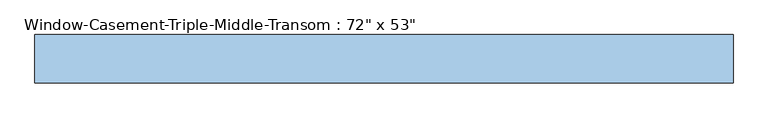
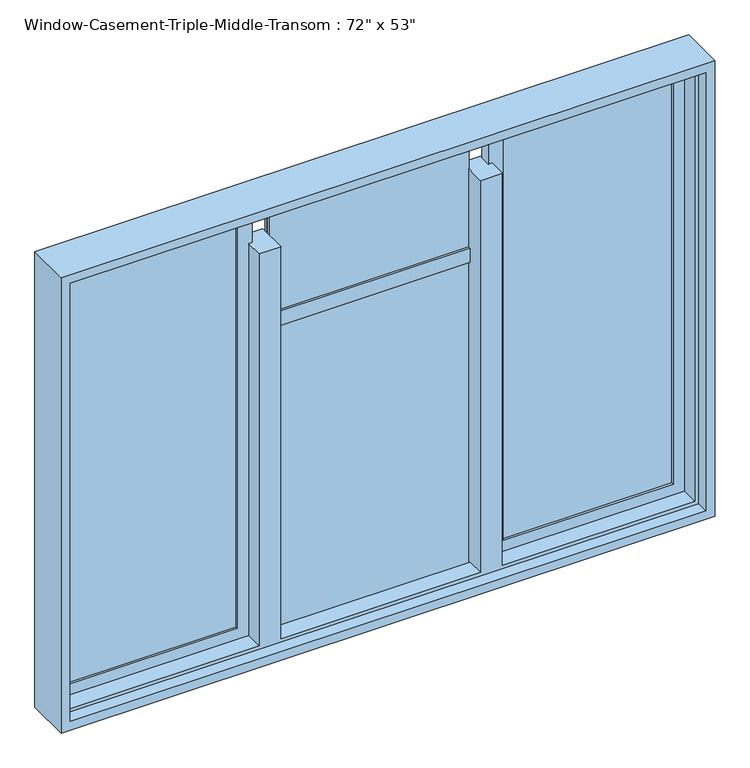
"""IFC4 building model written with IfcOpenShell, lengths in millimetres: window geometry."""

from ifc_helpers import new_model, si_unit, frame, origin, place, context, project, spatial, polyline, outline, extrude, faceted_brep, source, transform, mapped, element, save


def window_d2cb8397(model_context):
    return source(origin(), model_context, "Body", "SolidModel", [
        extrude(outline(polyline([(2235.2, 330.2), (939.8, 330.2), (939.8, 889.0), (2235.2, 889.0), (2235.2, 330.2)]), holes=[polyline([(2193.3296875, 847.1296875), (981.6703125, 847.1296875), (981.6703125, 372.0703125), (2193.3296875, 372.0703125), (2193.3296875, 847.1296875)])]), frame((0.0, 22.225, 0.0), z_axis=(0.0, 1.0, 0.0), x_axis=(0.0, 0.0, 1.0)), (0.0, 0.0, 1.0), 31.75),
        extrude(outline(polyline([(2235.2, -889.0), (939.8, -889.0), (939.8, -330.2), (2235.2, -330.2), (2235.2, -889.0)]), holes=[polyline([(2193.3296875, -372.0703125), (981.6703125, -372.0703125), (981.6703125, -847.1296875), (2193.3296875, -847.1296875), (2193.3296875, -372.0703125)])]), frame((0.0, 22.225, 0.0), z_axis=(0.0, 1.0, 0.0), x_axis=(0.0, 0.0, 1.0)), (0.0, 0.0, 1.0), 31.75),
        extrude(outline(polyline([(-372.0703125, 47.625), (-372.0703125, 41.275), (-847.1296875, 41.275), (-847.1296875, 47.625), (-372.0703125, 47.625)])), frame((0.0, 0.0, 949.9203125), z_axis=(0.0, 0.0, 1.0), x_axis=(1.0, 0.0, 0.0)), (0.0, 0.0, 1.0), 1275.159375),
        extrude(outline(polyline([(-372.0703125, 34.925), (-372.0703125, 28.575), (-847.1296875, 28.575), (-847.1296875, 34.925), (-372.0703125, 34.925)])), frame((0.0, 0.0, 949.9203125), z_axis=(0.0, 0.0, 1.0), x_axis=(1.0, 0.0, 0.0)), (0.0, 0.0, 1.0), 1275.159375),
        extrude(outline(polyline([(847.1296875, 47.625), (847.1296875, 41.275), (372.0703125, 41.275), (372.0703125, 47.625), (847.1296875, 47.625)])), frame((0.0, 0.0, 949.9203125), z_axis=(0.0, 0.0, 1.0), x_axis=(1.0, 0.0, 0.0)), (0.0, 0.0, 1.0), 1275.159375),
        extrude(outline(polyline([(847.1296875, 34.925), (847.1296875, 28.575), (372.0703125, 28.575), (372.0703125, 34.925), (847.1296875, 34.925)])), frame((0.0, 0.0, 949.9203125), z_axis=(0.0, 0.0, 1.0), x_axis=(1.0, 0.0, 0.0)), (0.0, 0.0, 1.0), 1275.159375),
        extrude(outline(polyline([(279.4, 53.975), (279.4, 22.225), (-279.4, 22.225), (-279.4, 53.975), (279.4, 53.975)])), frame((0.0, 0.0, 1835.8048438), z_axis=(0.0, 0.0, 1.0), x_axis=(1.0, 0.0, 0.0)), (0.0, 0.0, 1.0), 41.8703125),
        extrude(outline(polyline([(279.4, 47.625), (279.4, 41.275), (-279.4, 41.275), (-279.4, 47.625), (279.4, 47.625)])), frame((0.0, 0.0, 939.8), z_axis=(0.0, 0.0, 1.0), x_axis=(1.0, 0.0, 0.0)), (0.0, 0.0, 1.0), 896.0048437),
        extrude(outline(polyline([(279.4, 34.925), (279.4, 28.575), (-279.4, 28.575), (-279.4, 34.925), (279.4, 34.925)])), frame((0.0, 0.0, 939.8), z_axis=(0.0, 0.0, 1.0), x_axis=(1.0, 0.0, 0.0)), (0.0, 0.0, 1.0), 896.0048437),
        extrude(outline(polyline([(279.4, 47.625), (279.4, 41.275), (-279.4, 41.275), (-279.4, 47.625), (279.4, 47.625)])), frame((0.0, 0.0, 1877.6751563), z_axis=(0.0, 0.0, 1.0), x_axis=(1.0, 0.0, 0.0)), (0.0, 0.0, 1.0), 357.5248438),
        extrude(outline(polyline([(279.4, 34.925), (279.4, 28.575), (-279.4, 28.575), (-279.4, 34.925), (279.4, 34.925)])), frame((0.0, 0.0, 1877.6751563), z_axis=(0.0, 0.0, 1.0), x_axis=(1.0, 0.0, 0.0)), (0.0, 0.0, 1.0), 357.5248438),
        faceted_brep([(-889.0, 22.225, 2235.2), (-889.0, 63.5, 2235.2), (889.0, 63.5, 2235.2), (889.0, 22.225, 2235.2), (-878.8796875, -28.575, 2225.0796875), (-878.8796875, 22.225, 2225.0796875), (878.8796875, 22.225, 2225.0796875), (878.8796875, -28.575, 2225.0796875), (-889.0, -63.5, 2235.2), (-889.0, -28.575, 2235.2), (889.0, -28.575, 2235.2), (889.0, -63.5, 2235.2), (-914.4, 63.5, 2260.6), (-914.4, -63.5, 2260.6), (914.4, -63.5, 2260.6), (914.4, 63.5, 2260.6), (889.0, 63.5, 939.8), (889.0, 22.225, 939.8), (878.8796875, 22.225, 949.9203125), (878.8796875, -28.575, 949.9203125), (889.0, -28.575, 939.8), (889.0, -63.5, 939.8), (914.4, -63.5, 914.4), (914.4, 63.5, 914.4), (330.2, 22.225, 939.8), (-889.0, 63.5, 939.8), (-889.0, 22.225, 939.8), (-330.2, 22.225, 939.8), (-330.2, 60.325, 939.8), (-279.4, 60.325, 939.8), (-279.4, 22.225, 939.8), (279.4, 22.225, 939.8), (279.4, 60.325, 939.8), (330.2, 60.325, 939.8), (340.3203125, 22.225, 949.9203125), (340.3203125, -28.575, 949.9203125), (-878.8796875, 22.225, 949.9203125), (-878.8796875, -28.575, 949.9203125), (-340.3203125, -28.575, 949.9203125), (-340.3203125, 22.225, 949.9203125), (279.4, 22.225, 949.9203125), (-279.4, 22.225, 949.9203125), (-279.4, -28.575, 949.9203125), (279.4, -28.575, 949.9203125), (-889.0, -28.575, 939.8), (-889.0, -63.5, 939.8), (-914.4, -63.5, 914.4), (-914.4, 63.5, 914.4), (330.2, 22.225, 2108.2), (340.3203125, 22.225, 2108.2), (-340.3203125, 22.225, 2108.2), (-330.2, 22.225, 2108.2), (-279.4, 60.325, 2108.2), (-330.2, 60.325, 2108.2), (-340.3203125, -28.575, 2108.2), (-279.4, -28.575, 2108.2), (330.2, 60.325, 2108.2), (279.4, 60.325, 2108.2), (279.4, -28.575, 2108.2), (340.3203125, -28.575, 2108.2)], [[[0, 1, 2, 3]], [[4, 5, 6, 7]], [[8, 9, 10, 11]], [[12, 13, 14, 15]], [[3, 2, 16, 17]], [[7, 6, 18, 19]], [[11, 10, 20, 21]], [[15, 14, 22, 23]], [[24, 17, 16, 25, 26, 27, 28, 29, 30, 31, 32, 33]], [[19, 18, 34, 35]], [[36, 37, 38, 39]], [[40, 41, 42, 43]], [[21, 20, 44, 45]], [[23, 22, 46, 47]], [[1, 0, 26, 25]], [[0, 3, 17, 24, 48, 49, 34, 18, 6, 5, 36, 39, 50, 51, 27, 26]], [[41, 40, 31, 30]], [[5, 4, 37, 36]], [[9, 8, 45, 44]], [[14, 13, 46, 22], [8, 11, 21, 45]], [[13, 12, 47, 46]], [[12, 15, 23, 47], [2, 1, 25, 16]], [[52, 53, 51, 50, 54, 55]], [[56, 57, 58, 59, 49, 48]], [[53, 52, 29, 28]], [[27, 51, 53, 28]], [[52, 55, 42, 41, 30, 29]], [[57, 56, 33, 32]], [[58, 57, 32, 31, 40, 43]], [[56, 48, 24, 33]], [[54, 50, 39, 38]], [[49, 59, 35, 34]], [[10, 9, 44, 20], [4, 7, 19, 35, 59, 58, 43, 42, 55, 54, 38, 37]]]),
    ])


if __name__ == "__main__":
    model = new_model("IFC4")
    model_context = context("Model", 3, world=origin())
    ifc_project = project(units=[si_unit("LENGTHUNIT", "METRE", prefix="MILLI")], contexts=[model_context])
    site = spatial("IfcSite", under=ifc_project)
    building = spatial("IfcBuilding", under=site)
    placement = place(None, origin())
    window_shape = window_d2cb8397(model_context)
    element("IfcWindow", 1, ObjectType="Window-Casement-Triple-Middle-Transom : 72\" x 53\"", at=placement, inside=building, context=model_context, shape_type="MappedRepresentation", body=[
        mapped(window_shape, transform((0.0, 0.0, 0.0), x_axis=(1.0, 0.0, 0.0), y_axis=(0.0, 1.0, 0.0), z_axis=(0.0, 0.0, 1.0))),
    ])
    save(model, "model.ifc")

# Revit data of these elements
# Type "Window-Casement-Triple-Middle-Transom : 72\" x 53\""
#   Type Mark = "52"
#   Fire Rating = "0.5h"
#   Assembly Code = "B2020100"
#   Analytic Construction = "Double glazing - domestic"
#   Window Width = 2' - 0"
#   Window Inset [instance default] = 0' - 0 5/8"
#   Wall Thickness [instance default] = 0' - 6"
#   Visual Light Transmittance = 0.81
#   Transom Height Ratio = 0.3
#   Thermal Resistance (R) = 0.319569 (m²·K)/W
#   Solar Heat Gain Coefficient = 0.76
#   Rough Width = 6' - 0 1/2"
#   Rough Height = 4' - 5 1/2"
#   Heat Transfer Coefficient (U) = 3.12929 W/(m²·K)
#   Height = 4' - 5"
#   Transom Height = 1' - 3.9"
#   Frame Gap 3 [instance default] = 0' - 1 83/128"
#   Frame Gap 2 [instance default] = 0' - 0 5/8"
#   Frame Gap 1 = 0' - 1 51/128"
#   Default Sill Height = 3' - 0"
#   Width = 6' - 0"
#   Frame Material = Metal - Aluminum
#   Glass Panel Material = Glass
#   Wall Closure = (empty or 0)
# Element 1 (IfcWindow, "Window-Casement-Triple-Middle-Transom : 72\" x 53\"")
#   Wall Thickness = 0' - 5"
#   Materials on its faces: "Metal - Aluminum", "Glass"
# Materials
#   "Metal - Aluminum": class "Metal", colour RGB 247 247 247, transparency 0
#   "Glass": class "Glass", colour RGB 0 128 192, transparency 0.9, Description = "Soda Lime Glass", Cost = 0
